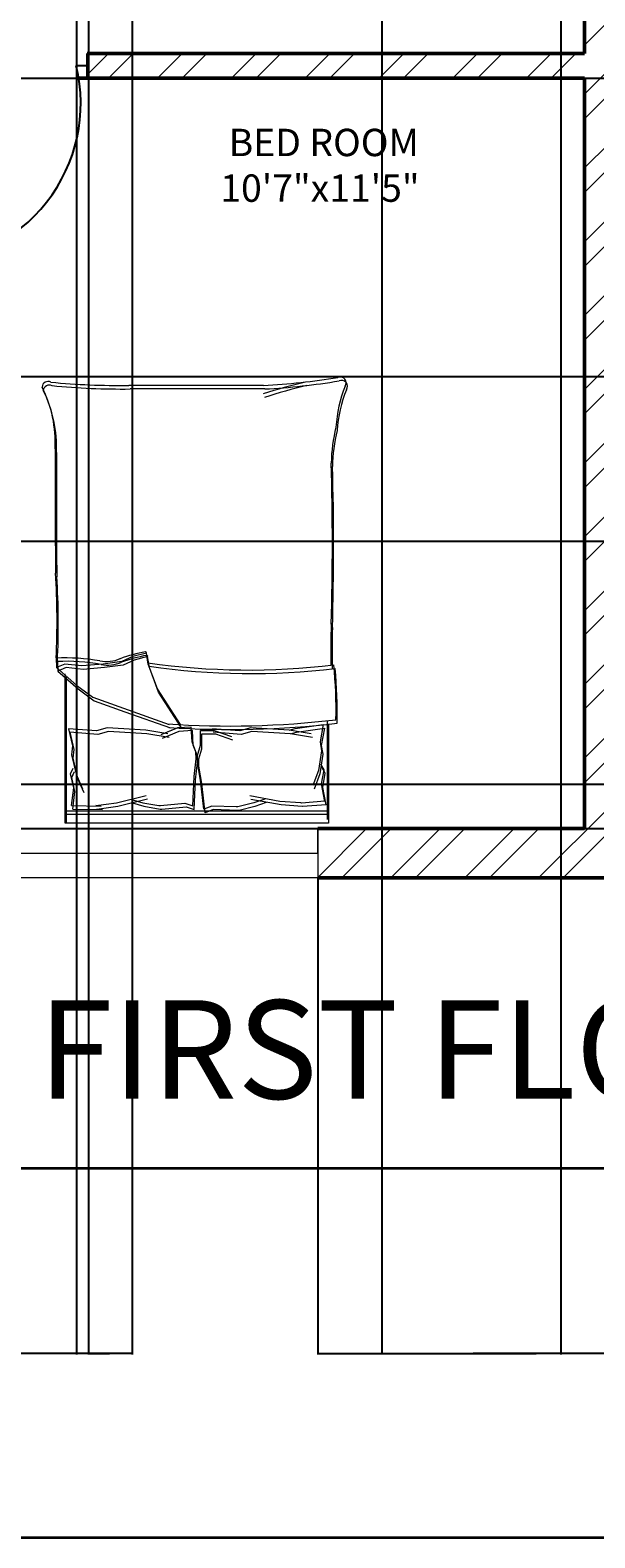
# Model space of a CAD drawing. Units: inches. Extents: x 2310 to 2937, y 1113 to 2410.
# Tile 2 of 23: x 2506 to 2609, y 1616 to 1891. Entities that reach past the tile are written whole.
import ezdxf

# ---------------------------------------------------------------- set-up
doc = ezdxf.new("R2010")
doc.units = ezdxf.units.IN
for name, color, linetype, lineweight in [('A-ANNO-DIMS', 2, 'Continuous', 18), ('A-ANNO-TTLB', 7, 'Continuous', 35), ('A-AREA-IDEN', 7, 'Continuous', 18), ('A-DOOR', 31, 'Continuous', 25), ('A-FURN', 8, 'Continuous', 18), ('A-GLAZ', 191, 'Continuous', 20), ('A-WALL', 7, 'Continuous', 50), ('A-WALL-PATT', 85, 'Continuous', 13)]:
    doc.layers.add(name, color=color, linetype=linetype, lineweight=lineweight)
doc.styles.get("Standard").update_dxf_attribs({"font": 'arial.ttf'})
doc.dimstyles.get("Standard").update_dxf_attribs({"dimtxt": 0.18, "dimasz": 0.18, "dimexe": 0.18, "dimexo": 0.0625, "dimgap": 0.09, "dimtad": 0, "dimtih": 1, "dimtoh": 1, "dimdec": 4, "dimzin": 0, "dimdsep": 46, "dimtxsty": 'Standard', "dimcen": 0.09, "dimadec": 0, "dimazin": 0, "dimtfac": 1, "dimtdec": 4, "dimtofl": 0, "dimtmove": 0, "dimatfit": 3, "dimfxl": 1, "dimtolj": 1, "dimtzin": 0, "dimarcsym": 0})

# ---------------------------------------------------------------- blocks, each defined once
blk = doc.blocks.new('BED-DOUBLE')
for p, q in [((3.56, 63.44), (3.56, 81.55)), ((3.56, 63.44), (3.56, 81.55)), ((3.56, 81.55), (51.58, 81.55)), ((3.56, 80.01), (51.35, 80.01)), ((3.56, 80.01), (51.35, 80.01)), ((3.79, 62.8), (3.79, 80.91)), ((3.79, 62.8), (3.79, 80.91)), ((51.35, 81.55), (51.35, 54.94)), ((51.35, 81.55), (51.35, 54.94)), ((51.58, 81.55), (51.58, 80.91)), ((51.58, 80.91), (51.58, 54.3)), ((51.58, 80.91), (51.58, 54.3)), ((3.79, 79.38), (51.58, 79.38)), ((3.79, 79.38), (51.58, 79.38)), ((3.98, 78.21), (8.27, 78.54)), ((3.98, 78.23), (4.56, 75.05)), ((3.98, 78.23), (4.56, 75.05)), ((3.99, 78.21), (8.27, 78.54)), ((4.21, 77.57), (8.49, 77.9)), ((4.21, 77.57), (8.49, 77.9)), ((4.21, 77.59), (4.79, 74.41)), ((4.21, 77.59), (4.79, 74.41)), ((8.27, 78.54), (8.37, 78.52)), ((8.27, 78.54), (8.37, 78.52)), ((8.37, 78.52), (12.19, 78.23)), ((8.37, 78.52), (12.19, 78.23)), ((8.49, 77.9), (8.6, 77.88)), ((8.49, 77.9), (8.6, 77.88)), ((8.6, 77.88), (12.42, 77.59)), ((8.6, 77.88), (12.42, 77.59)), ((12.19, 78.23), (17.69, 77.22)), ((12.19, 78.23), (17.69, 77.22)), ((12.42, 77.59), (17.92, 76.58)), ((12.42, 77.59), (17.92, 76.58)), ((14.94, 77.8), (16.97, 78.52)), ((14.94, 77.8), (16.96, 78.52)), ((15.17, 77.16), (17.19, 77.88)), ((15.17, 77.16), (17.19, 77.88)), ((16.96, 78.52), (19.86, 79.24)), ((16.97, 78.52), (19.86, 79.24)), ((17.19, 77.88), (20.08, 78.61)), ((17.19, 77.88), (20.08, 78.61)), ((19.86, 79.24), (20.18, 79.24)), ((19.86, 79.24), (20.18, 79.24)), ((20.08, 78.61), (20.41, 78.61)), ((20.08, 78.61), (20.41, 78.61)), ((20.18, 79.24), (24.62, 79.1)), ((20.18, 79.24), (24.62, 79.1)), ((20.41, 78.61), (24.85, 78.46)), ((20.41, 78.61), (24.85, 78.46)), ((24.62, 79.1), (26.07, 79.68)), ((24.62, 79.1), (26.07, 79.68)), ((24.85, 78.46), (26.3, 79.04)), ((24.85, 78.46), (26.3, 79.04)), ((26.07, 79.68), (26.65, 74.33)), ((26.07, 79.68), (26.65, 74.33)), ((26.3, 79.04), (26.88, 73.69)), ((26.3, 79.04), (26.88, 73.69)), ((28.06, 79.06), (27.82, 73.68)), ((28.06, 79.06), (27.82, 73.68)), ((28.29, 78.42), (28.05, 73.04)), ((28.29, 78.42), (28.05, 73.04)), ((29.54, 78.57), (28.06, 79.06)), ((29.54, 78.57), (28.06, 79.06)), ((29.77, 77.93), (28.29, 78.42)), ((29.77, 77.93), (28.29, 78.42)), ((33.97, 78.99), (29.54, 78.57)), ((33.97, 78.99), (29.54, 78.57)), ((34.2, 78.35), (29.77, 77.93)), ((34.2, 78.35), (29.77, 77.93)), ((34.29, 79.01), (33.97, 78.99)), ((34.29, 79.01), (33.97, 78.99)), ((34.52, 78.37), (34.2, 78.35)), ((34.52, 78.37), (34.2, 78.35)), ((37.22, 78.47), (34.29, 79.01)), ((37.22, 78.47), (34.29, 79.01)), ((37.45, 77.83), (34.52, 78.37)), ((37.45, 77.83), (34.52, 78.37)), ((42, 78.48), (36.58, 77.13)), ((42, 78.48), (36.58, 77.13)), ((42.23, 77.84), (36.81, 76.49)), ((42.23, 77.84), (36.81, 76.49)), ((39.29, 77.87), (37.22, 78.47)), ((39.29, 77.87), (37.22, 78.47)), ((39.52, 77.24), (37.45, 77.83)), ((39.51, 77.24), (37.45, 77.83)), ((45.8, 79.01), (42, 78.48)), ((45.8, 79.01), (42, 78.48)), ((46.03, 78.37), (42.23, 77.84)), ((46.03, 78.37), (42.23, 77.84)), ((50.2, 78.99), (44.8, 79.09)), ((44.8, 79.09), (45.8, 79.01)), ((50.2, 78.99), (44.8, 79.09)), ((44.8, 79.09), (45.8, 79.01)), ((50.43, 78.35), (45.02, 78.45)), ((45.02, 78.45), (46.03, 78.37)), ((50.43, 78.35), (45.02, 78.45)), ((45.02, 78.45), (46.03, 78.37)), ((50.2, 78.99), (49.82, 75.78)), ((50.2, 78.99), (49.82, 75.78)), ((50.43, 78.35), (50.05, 75.14)), ((50.43, 78.35), (50.05, 75.14)), ((4.56, 75.05), (4.13, 72.45)), ((4.56, 75.05), (4.13, 72.45)), ((4.79, 74.41), (4.35, 71.81)), ((4.79, 74.41), (4.35, 71.81)), ((5.14, 72.59), (6.15, 75.34)), ((5.14, 72.59), (6.15, 75.34)), ((5.37, 71.95), (6.38, 74.7)), ((5.37, 71.95), (6.38, 74.7)), ((26.65, 74.33), (27.23, 71.15)), ((26.65, 74.33), (27.23, 71.15)), ((49.4, 73.29), (48.21, 75.97)), ((49.4, 73.29), (48.21, 75.97)), ((49.62, 72.65), (48.44, 75.33)), ((49.62, 72.65), (48.44, 75.33)), ((49.82, 75.78), (50.42, 73.21)), ((49.82, 75.78), (50.41, 73.21)), ((50.05, 75.14), (50.64, 72.57)), ((50.05, 75.14), (50.64, 72.57)), ((4.13, 72.45), (4.7, 71.44)), ((4.13, 72.45), (4.7, 71.44)), ((4.35, 71.81), (4.93, 70.8)), ((4.35, 71.81), (4.93, 70.8)), ((4.56, 68.98), (5.14, 72.59)), ((4.56, 68.98), (5.14, 72.59)), ((4.79, 68.34), (5.37, 71.95)), ((4.79, 68.34), (5.37, 71.95)), ((26.88, 73.69), (27.45, 70.51)), ((26.88, 73.69), (27.45, 70.51)), ((27.82, 73.68), (27.44, 70.47)), ((27.82, 73.68), (27.44, 70.47)), ((28.05, 73.04), (27.67, 69.83)), ((28.05, 73.04), (27.67, 69.83)), ((50.2, 69.72), (49.4, 73.29)), ((50.2, 69.72), (49.4, 73.29)), ((50.43, 69.08), (49.62, 72.65)), ((50.43, 69.08), (49.62, 72.65)), ((50.42, 73.21), (49.9, 72.16)), ((50.41, 73.21), (49.9, 72.16)), ((50.64, 72.57), (50.13, 71.52)), ((50.64, 72.57), (50.13, 71.52)), ((4.85, 67.39), (4.56, 68.98)), ((4.85, 67.39), (4.56, 68.98)), ((27.23, 69.85), (26.65, 67.97)), ((27.23, 69.85), (26.65, 67.97)), ((27.45, 69.21), (26.88, 67.33)), ((27.45, 69.21), (26.88, 67.33)), ((27.23, 71.15), (27.23, 69.85)), ((27.23, 71.15), (27.23, 69.85)), ((27.44, 70.47), (27.52, 69.17)), ((27.44, 70.47), (27.52, 69.17)), ((27.45, 70.51), (27.45, 69.21)), ((27.45, 70.51), (27.45, 69.21)), ((27.52, 69.17), (28.22, 67.33)), ((27.52, 69.17), (28.22, 67.33)), ((27.67, 69.83), (27.75, 68.53)), ((27.67, 69.83), (27.75, 68.53)), ((50.01, 68.11), (50.2, 69.72)), ((50.01, 68.11), (50.2, 69.72)), ((50.24, 67.48), (50.43, 69.08)), ((50.24, 67.48), (50.43, 69.08)), ((4.27, 64.21), (4.85, 67.39)), ((4.27, 64.21), (4.85, 67.39)), ((4.5, 63.57), (5.08, 66.75)), ((4.5, 63.57), (5.08, 66.75)), ((5.08, 66.75), (4.79, 68.34)), ((5.08, 66.75), (4.79, 68.34)), ((24.19, 65.29), (21.04, 66.38)), ((24.19, 65.29), (21.05, 66.38)), ((26.65, 67.97), (26.65, 65.29)), ((26.65, 67.97), (26.65, 65.29)), ((26.88, 67.33), (26.88, 64.65)), ((26.88, 67.33), (26.88, 64.65)), ((27.75, 68.53), (28.45, 66.69)), ((27.75, 68.53), (28.44, 66.69)), ((28.22, 67.33), (28.38, 64.66)), ((28.22, 67.33), (28.38, 64.66)), ((28.44, 66.69), (28.61, 64.02)), ((28.45, 66.69), (28.61, 64.02)), ((30.84, 64.81), (33.91, 66.09)), ((30.84, 64.81), (33.91, 66.09)), ((50.78, 64.98), (50.01, 68.11)), ((50.78, 64.98), (50.01, 68.11)), ((51.01, 64.34), (50.24, 67.48)), ((51.01, 64.34), (50.24, 67.48)), ((9.37, 64.93), (4.27, 64.21)), ((9.37, 64.93), (4.27, 64.21)), ((9.6, 64.29), (4.5, 63.57)), ((9.6, 64.29), (4.5, 63.57)), ((6.47, 65.92), (10.5, 65.25)), ((6.47, 65.92), (10.5, 65.25)), ((6.7, 65.28), (10.73, 64.61)), ((6.7, 65.28), (10.73, 64.61)), ((10.5, 65.25), (9.37, 64.93)), ((10.5, 65.25), (9.37, 64.93)), ((10.73, 64.61), (9.6, 64.29)), ((10.73, 64.61), (9.6, 64.29)), ((10.5, 65.25), (17.51, 64.82)), ((10.5, 65.25), (17.51, 64.82)), ((10.73, 64.61), (17.74, 64.18)), ((10.73, 64.61), (17.74, 64.18)), ((17.51, 64.82), (19.47, 65.38)), ((17.51, 64.82), (19.47, 65.38)), ((17.74, 64.18), (19.7, 64.74)), ((17.74, 64.18), (19.7, 64.74)), ((19.47, 65.38), (24.6, 64.98)), ((19.47, 65.38), (24.6, 64.98)), ((19.7, 64.74), (24.83, 64.34)), ((19.7, 64.74), (24.83, 64.34)), ((24.42, 64.65), (21.27, 65.74)), ((24.42, 64.65), (21.27, 65.74)), ((26.65, 65.29), (24.19, 65.29)), ((26.65, 65.29), (24.19, 65.29)), ((26.88, 64.65), (24.42, 64.65)), ((26.88, 64.65), (24.42, 64.65)), ((28.38, 64.66), (30.84, 64.81)), ((28.38, 64.66), (30.84, 64.81)), ((28.61, 64.02), (31.07, 64.17)), ((28.61, 64.02), (31.06, 64.17)), ((30.35, 64.17), (34.54, 57.67)), ((30.35, 64.17), (34.54, 57.67)), ((30.57, 63.53), (34.76, 57.03)), ((30.57, 63.53), (34.76, 57.03)), ((31.06, 64.17), (34.14, 65.45)), ((31.07, 64.17), (34.14, 65.45)), ((40.73, 61.23), (32.39, 64.17)), ((40.73, 61.23), (32.39, 64.17)), ((40.96, 60.59), (32.62, 63.53)), ((40.96, 60.59), (32.62, 63.53)), ((32.65, 65.92), (36.68, 65.25)), ((32.65, 65.92), (36.68, 65.25)), ((32.88, 65.28), (36.91, 64.61)), ((32.88, 65.28), (36.91, 64.61)), ((36.68, 65.25), (43.69, 64.82)), ((36.68, 65.25), (43.69, 64.82)), ((36.91, 64.61), (43.92, 64.18)), ((36.91, 64.61), (43.92, 64.18)), ((43.69, 64.82), (45.65, 65.38)), ((43.69, 64.82), (45.65, 65.38)), ((43.92, 64.18), (45.88, 64.74)), ((43.92, 64.18), (45.88, 64.74)), ((45.65, 65.38), (50.78, 64.98)), ((45.65, 65.38), (50.78, 64.98)), ((45.88, 64.74), (51.01, 64.34)), ((45.88, 64.74), (51.01, 64.34)), ((46.31, 59.22), (40.73, 61.23)), ((46.31, 59.22), (40.73, 61.23)), ((46.53, 58.58), (40.96, 60.59)), ((46.53, 58.58), (40.96, 60.59)), ((49.25, 57.05), (46.31, 59.22)), ((49.25, 57.05), (46.31, 59.22)), ((49.48, 56.41), (46.53, 58.58)), ((49.48, 56.41), (46.53, 58.58)), ((34.54, 57.67), (36.24, 53.18)), ((34.54, 57.67), (36.24, 53.18)), ((34.76, 57.03), (36.47, 52.54)), ((34.76, 57.03), (36.47, 52.54)), ((52.95, 53.8), (49.25, 57.05)), ((52.95, 53.8), (49.25, 57.05)), ((53.18, 53.16), (49.48, 56.41)), ((53.18, 53.16), (49.48, 56.41)), ((36.24, 53.18), (36.55, 51.17)), ((36.24, 53.18), (36.55, 51.17)), ((36.47, 52.54), (36.78, 50.53)), ((36.47, 52.54), (36.78, 50.53)), ((39.03, 51.79), (41.04, 52.72)), ((39.03, 51.79), (41.04, 52.72)), ((41.04, 52.72), (44.45, 53.18)), ((41.04, 52.72), (44.45, 53.18)), ((41.27, 52.08), (44.68, 52.54)), ((41.27, 52.08), (44.68, 52.54)), ((44.45, 53.18), (48.32, 53.49)), ((44.45, 53.18), (48.32, 53.49)), ((44.68, 52.54), (48.55, 52.85)), ((44.68, 52.54), (48.55, 52.85)), ((48.32, 53.49), (51.42, 53.18)), ((48.32, 53.49), (51.42, 53.18)), ((48.55, 52.85), (51.65, 52.54)), ((48.55, 52.85), (51.65, 52.54)), ((51.42, 53.18), (52.95, 53.8)), ((51.42, 53.18), (52.95, 53.8)), ((51.65, 52.54), (53.18, 53.16)), ((51.65, 52.54), (53.18, 53.16)), ((53.03, 52.06), (52.95, 53.8, 3.87)), ((53.03, 52.06), (52.95, 53.8, 3.87)), ((53.26, 51.42), (53.18, 53.16, 3.87)), ((53.26, 51.42), (53.18, 53.16, 3.87)), ((36.55, 51.17), (39.03, 51.79)), ((36.55, 51.17), (39.03, 51.79)), ((36.78, 50.53), (39.26, 51.15)), ((36.78, 50.53), (39.26, 51.15)), ((39.26, 51.15), (41.27, 52.08)), ((39.26, 51.15), (41.27, 52.08)), ((15.15, 2.3), (39.76, 2.3)), ((15.15, 2.3), (39.76, 2.3)), ((15.38, 1.66), (39.99, 1.66)), ((15.38, 1.66), (39.99, 1.66))]:
    blk.add_line(p, q)
for centre, radius, start, end in [((85.25, 61.45), 83.31, 178.7218, 185.604), ((85.25, 61.45), 83.31, 178.7218, 185.604), ((21.45, -100.5), 164.97, 86.0865, 96.7821), ((21.45, -100.5), 164.97, 86.0865, 96.7821), ((21.67, -101.14), 164.97, 86.0865, 96.7821), ((21.67, -101.14), 164.97, 86.0865, 96.7821), ((85.48, 60.81), 83.31, 178.7218, 185.604), ((85.48, 60.81), 83.31, 178.7218, 185.604), ((17.84, -74.77), 129.02, 81.7845, 96.9006), ((17.84, -74.77), 129.02, 81.7845, 96.9006), ((18.07, -75.41), 129.02, 81.7845, 96.9006), ((18.07, -75.41), 129.02, 81.7845, 96.9006), ((-167.22, 50.37), 170.11, 358.4762, 1.0082), ((-167.22, 50.37), 170.11, 358.4762, 1.0082), ((-166.99, 49.74), 170.11, 358.4762, 1.0082), ((-166.99, 49.74), 170.11, 358.4762, 1.0082), ((43.83, 46.48), 6.22, 78.6608, 113.7384), ((43.83, 46.48), 6.22, 78.6608, 113.7384), ((51.41, 88.2), 36.18, 259.8763, 272.5657), ((51.41, 88.2), 36.18, 259.8763, 272.5657), ((36.72, 51.11), 0.185, 160.2464, 271.1377), ((36.72, 51.11), 0.185, 160.2464, 271.1377), ((31.24, 80.07), 29.65, 280.6617, 289.8806), ((31.24, 80.07), 29.65, 280.6617, 289.8806), ((36.95, 50.47), 0.185, 160.2464, 271.1377), ((36.95, 50.47), 0.185, 160.2464, 271.1377), ((31.47, 79.43), 29.65, 280.6617, 289.8806), ((31.47, 79.43), 29.65, 280.6617, 289.8806), ((44.06, 45.84), 6.22, 78.6608, 113.7384), ((44.06, 45.84), 6.22, 78.6608, 113.7384), ((51.64, 87.57), 36.18, 259.8763, 272.5657), ((51.64, 87.57), 36.18, 259.8763, 272.5657), ((182.35, 45.23), 129.5, 176.9791, 183.8365), ((182.35, 45.23), 129.5, 176.9791, 183.8365), ((182.58, 44.59), 129.5, 176.9791, 183.8365), ((182.58, 44.59), 129.5, 176.9791, 183.8365), ((484.91, 30.93), 482.31, 178.2277, 181.7185), ((484.91, 30.93), 482.31, 178.2277, 181.7185), ((485.14, 30.3), 482.31, 178.2277, 181.7185), ((485.14, 30.3), 482.31, 178.2277, 181.7185), ((-4508.66, 13.73), 4561.86, 0.00217, 0.28689), ((-4508.66, 13.73), 4561.86, 0.00217, 0.28689), ((-4508.43, 13.09), 4561.86, 0.00217, 0.28689), ((-4508.43, 13.09), 4561.86, 0.00217, 0.28689), ((-26.81, 17.03), 29.63, 346.0648, 358.9113), ((-26.81, 17.03), 29.63, 346.0648, 358.9113), ((-26.58, 16.39), 29.63, 346.0648, 358.9113), ((-26.58, 16.39), 29.63, 346.0648, 358.9113), ((76.24, 12.88), 23.07, 177.4714, 206.4681), ((76.24, 12.88), 23.07, 177.4714, 206.4681), ((76.47, 12.24), 23.07, 177.4714, 206.4681), ((76.47, 12.24), 23.07, 177.4714, 206.4681), ((-21.57, 11.27), 23.56, 337.9751, 356.652), ((-21.57, 11.27), 23.56, 337.9751, 356.652), ((-21.34, 10.63), 23.56, 337.9751, 356.652), ((-21.34, 10.63), 23.56, 337.9751, 356.652), ((-17.14, 105.26), 106.46, 283.3832, 287.7053), ((-17.14, 105.26), 106.46, 283.3832, 287.7053), ((-16.91, 104.62), 106.46, 283.3832, 287.7053), ((-16.91, 104.62), 106.46, 283.3832, 287.7053), ((1.17, 1.83), 1.09, 146.1736, 293.4781), ((1.17, 1.83), 1.09, 146.1736, 293.4781), ((1.4, 1.19), 1.09, 146.1736, 293.4781), ((1.4, 1.19), 1.09, 146.1736, 293.4781), ((21.51, -119.29), 121.76, 92.9958, 99.4091), ((21.51, -119.29), 121.76, 92.9958, 99.4091), ((21.74, -119.93), 121.76, 92.9958, 99.4091), ((21.74, -119.93), 121.76, 92.9958, 99.4091), ((41.24, -130.73), 133.04, 84.4998, 90.6351), ((41.24, -130.73), 133.04, 84.4998, 90.6351), ((41.47, -131.37), 133.04, 84.4998, 90.6351), ((41.47, -131.37), 133.04, 84.4998, 90.6351), ((54.5, 2.68), 1.1, 242.6588, 356.02), ((54.5, 2.68), 1.1, 242.6588, 356.02), ((54.72, 2.04), 1.1, 242.6588, 356.02), ((54.72, 2.04), 1.1, 242.6588, 356.02)]:
    blk.add_arc(centre, radius, start, end)
blk = doc.blocks.new('WIN-60IN')
for p, q in [((4.5, 60), (0, 60)), ((0, 60), (9, 60)), ((0, 60), (0, 0)), ((4.5, 0), (4.5, 60)), ((9, 60), (9, 0)), ((0, 0), (9, 0)), ((9, 0), (4.5, 0))]:
    blk.add_line(p, q)
blk = doc.blocks.new('*D44')
at = {"layer": 'A-ANNO-DIMS', "color": 0, "lineweight": -2, "transparency": 16777216}
for p, q in [((2558.31, 1736.45), (2558.31, 1649.5)), ((2638.89, 1736.45), (2638.89, 1649.5)), ((2558.49, 1649.68), (2598.21, 1649.68)), ((2638.71, 1649.68), (2598.99, 1649.68))]:
    blk.add_line(p, q, dxfattribs=at)
at = {"layer": 'A-ANNO-DIMS', "color": 0, "transparency": 16777216}
for points in [[(2558.49, 1649.71), (2558.49, 1649.65), (2558.31, 1649.68)], [(2638.71, 1649.71), (2638.71, 1649.65), (2638.89, 1649.68)]]:
    blk.add_solid(points, dxfattribs=at)
at = {"layer": 'Defpoints', "color": 0, "transparency": 16777216}
for p in [(2558.31, 1736.51), (2638.89, 1736.51), (2638.89, 1649.68)]:
    blk.add_point(p, dxfattribs=at)
at = {"layer": 'A-ANNO-DIMS', "color": 0, "transparency": 16777216, "insert": (2598.6, 1649.68), "char_height": 0.18, "attachment_point": 5}
blk.add_mtext('\\A1;80.59', dxfattribs=at)
blk = doc.blocks.new('*D55')
at = {"layer": 'A-ANNO-DIMS', "color": 0, "lineweight": -2, "transparency": 16777216}
for p, q in [((2403.55, 1753.64), (2858.02, 1753.64)), ((2857.84, 1753.46), (2857.84, 1749.76)), ((2857.84, 1745.69), (2857.84, 1749.4)), ((2403.55, 1745.51), (2858.02, 1745.51))]:
    blk.add_line(p, q, dxfattribs=at)
at = {"layer": 'A-ANNO-DIMS', "color": 0, "transparency": 16777216}
for points in [[(2857.81, 1753.46), (2857.87, 1753.46), (2857.84, 1753.64)], [(2857.81, 1745.69), (2857.87, 1745.69), (2857.84, 1745.51)]]:
    blk.add_solid(points, dxfattribs=at)
at = {"layer": 'Defpoints', "color": 0, "transparency": 16777216}
for p in [(2403.49, 1753.64), (2857.84, 1753.64), (2403.49, 1745.51)]:
    blk.add_point(p, dxfattribs=at)
at = {"layer": 'A-ANNO-DIMS', "color": 0, "transparency": 16777216, "insert": (2857.84, 1749.58), "char_height": 0.18, "attachment_point": 5}
blk.add_mtext('\\A1;8.127', dxfattribs=at)
blk = doc.blocks.new('*D56')
at = {"layer": 'A-ANNO-DIMS', "color": 0, "lineweight": -2, "transparency": 16777216}
for p, q in [((2403.55, 1828.04), (2858.02, 1828.04)), ((2857.84, 1827.86), (2857.84, 1813.21)), ((2857.84, 1798.19), (2857.84, 1812.85)), ((2403.55, 1798.01), (2858.02, 1798.01))]:
    blk.add_line(p, q, dxfattribs=at)
at = {"layer": 'A-ANNO-DIMS', "color": 0, "transparency": 16777216}
for points in [[(2857.81, 1827.86), (2857.87, 1827.86), (2857.84, 1828.04)], [(2857.81, 1798.19), (2857.87, 1798.19), (2857.84, 1798.01)]]:
    blk.add_solid(points, dxfattribs=at)
at = {"layer": 'Defpoints', "color": 0, "transparency": 16777216}
for p in [(2403.49, 1828.04), (2857.84, 1828.04), (2403.49, 1798.01)]:
    blk.add_point(p, dxfattribs=at)
at = {"layer": 'A-ANNO-DIMS', "color": 0, "transparency": 16777216, "insert": (2857.84, 1813.03), "char_height": 0.18, "attachment_point": 5}
blk.add_mtext('\\A1;30.03', dxfattribs=at)
blk = doc.blocks.new('*D58')
at = {"layer": 'A-ANNO-DIMS', "color": 0, "lineweight": -2, "transparency": 16777216}
for p, q in [((2475.55, 1882.51), (2858.02, 1882.51)), ((2857.84, 1882.33), (2857.84, 1840.45)), ((2857.84, 1798.19), (2857.84, 1840.08)), ((2475.55, 1798.01), (2858.02, 1798.01))]:
    blk.add_line(p, q, dxfattribs=at)
at = {"layer": 'A-ANNO-DIMS', "color": 0, "transparency": 16777216}
for points in [[(2857.81, 1882.33), (2857.87, 1882.33), (2857.84, 1882.51)], [(2857.81, 1798.19), (2857.87, 1798.19), (2857.84, 1798.01)]]:
    blk.add_solid(points, dxfattribs=at)
at = {"layer": 'Defpoints', "color": 0, "transparency": 16777216}
for p in [(2475.49, 1882.51), (2857.84, 1882.51), (2475.49, 1798.01)]:
    blk.add_point(p, dxfattribs=at)
at = {"layer": 'A-ANNO-DIMS', "color": 0, "transparency": 16777216, "insert": (2857.84, 1840.26), "char_height": 0.18, "attachment_point": 5}
blk.add_mtext('\\A1;84.5', dxfattribs=at)
blk = doc.blocks.new('*D61')
at = {"layer": 'A-ANNO-DIMS', "color": 0, "lineweight": -2, "transparency": 16777216}
for p, q in [((2484.33, 2205.95), (2484.33, 1649.5)), ((2514.27, 2205.95), (2514.27, 1649.5)), ((2484.51, 1649.68), (2498.9, 1649.68)), ((2514.09, 1649.68), (2499.69, 1649.68))]:
    blk.add_line(p, q, dxfattribs=at)
at = {"layer": 'A-ANNO-DIMS', "color": 0, "transparency": 16777216}
for points in [[(2484.51, 1649.71), (2484.51, 1649.65), (2484.33, 1649.68)], [(2514.09, 1649.71), (2514.09, 1649.65), (2514.27, 1649.68)]]:
    blk.add_solid(points, dxfattribs=at)
at = {"layer": 'Defpoints', "color": 0, "transparency": 16777216}
for p in [(2484.33, 2206.01), (2514.27, 2206.01), (2514.27, 1649.68)]:
    blk.add_point(p, dxfattribs=at)
at = {"layer": 'A-ANNO-DIMS', "color": 0, "transparency": 16777216, "insert": (2499.3, 1649.68), "char_height": 0.18, "attachment_point": 5}
blk.add_mtext('\\A1;29.94', dxfattribs=at)
blk = doc.blocks.new('*D62')
at = {"layer": 'A-ANNO-DIMS', "color": 0, "lineweight": -2, "transparency": 16777216}
for p, q in [((2569.99, 2093.45), (2569.99, 1649.5)), ((2602.69, 2093.45), (2602.69, 1649.5)), ((2570.17, 1649.68), (2586.02, 1649.68)), ((2602.51, 1649.68), (2586.66, 1649.68))]:
    blk.add_line(p, q, dxfattribs=at)
at = {"layer": 'A-ANNO-DIMS', "color": 0, "transparency": 16777216}
for points in [[(2570.17, 1649.71), (2570.17, 1649.65), (2569.99, 1649.68)], [(2602.51, 1649.71), (2602.51, 1649.65), (2602.69, 1649.68)]]:
    blk.add_solid(points, dxfattribs=at)
at = {"layer": 'Defpoints', "color": 0, "transparency": 16777216}
for p in [(2569.99, 2093.51), (2602.69, 2093.51), (2602.69, 1649.68)]:
    blk.add_point(p, dxfattribs=at)
at = {"layer": 'A-ANNO-DIMS', "color": 0, "transparency": 16777216, "insert": (2586.34, 1649.68), "char_height": 0.18, "attachment_point": 5}
blk.add_mtext('\\A1;32.7', dxfattribs=at)
blk = doc.blocks.new('*D63')
at = {"layer": 'A-ANNO-DIMS', "color": 0, "lineweight": -2, "transparency": 16777216}
for p, q in [((2436.46, 1999.45), (2436.46, 1649.5)), ((2524.46, 1999.45), (2524.46, 1649.5)), ((2436.64, 1649.68), (2480.25, 1649.68)), ((2524.28, 1649.68), (2480.68, 1649.68))]:
    blk.add_line(p, q, dxfattribs=at)
at = {"layer": 'A-ANNO-DIMS', "color": 0, "transparency": 16777216}
for points in [[(2436.64, 1649.71), (2436.64, 1649.65), (2436.46, 1649.68)], [(2524.28, 1649.71), (2524.28, 1649.65), (2524.46, 1649.68)]]:
    blk.add_solid(points, dxfattribs=at)
at = {"layer": 'Defpoints', "color": 0, "transparency": 16777216}
for p in [(2436.46, 1999.51), (2524.46, 1999.51), (2524.46, 1649.68)]:
    blk.add_point(p, dxfattribs=at)
at = {"layer": 'A-ANNO-DIMS', "color": 0, "transparency": 16777216, "insert": (2480.46, 1649.68), "char_height": 0.18, "attachment_point": 5}
blk.add_mtext('\\A1;88', dxfattribs=at)
blk = doc.blocks.new('*D66')
at = {"layer": 'A-ANNO-DIMS', "color": 0, "lineweight": -2, "transparency": 16777216}
for p, q in [((2516.46, 2093.45), (2516.46, 1649.5)), ((2524.46, 2093.45), (2524.46, 1649.5)), ((2516.64, 1649.68), (2520.32, 1649.68)), ((2524.28, 1649.68), (2520.61, 1649.68))]:
    blk.add_line(p, q, dxfattribs=at)
at = {"layer": 'A-ANNO-DIMS', "color": 0, "transparency": 16777216}
for points in [[(2516.64, 1649.71), (2516.64, 1649.65), (2516.46, 1649.68)], [(2524.28, 1649.71), (2524.28, 1649.65), (2524.46, 1649.68)]]:
    blk.add_solid(points, dxfattribs=at)
at = {"layer": 'Defpoints', "color": 0, "transparency": 16777216}
for p in [(2516.46, 2093.51), (2524.46, 2093.51), (2524.46, 1649.68)]:
    blk.add_point(p, dxfattribs=at)
at = {"layer": 'A-ANNO-DIMS', "color": 0, "transparency": 16777216, "insert": (2520.46, 1649.68), "char_height": 0.18, "attachment_point": 5}
blk.add_mtext('\\A1;8', dxfattribs=at)

msp = doc.modelspace()

# ---------------------------------------------------------------- hatches: boundary and pattern name
at = {"layer": 'A-WALL-PATT'}
h = msp.add_hatch(dxfattribs=at)
h.set_pattern_fill('ANSI32', color=256)
h.paths.add_polyline_path([(2639.1394, 2356.5139), (2563.662, 2356.5139), (2563.662, 2347.5139), (2606.9859, 2347.5139), (2606.9859, 2210.5139), (2514.2692, 2210.5139), (2514.2692, 2206.0139), (2606.9859, 2206.0139), (2606.9859, 2098.0139), (2602.689, 2098.0139), (2602.689, 2093.5139), (2615.5262, 2093.5139), (2615.5262, 2095.7639), (2615.5262, 2098.0139), (2611.4859, 2098.0139), (2611.4859, 2206.0139), (2703.9391, 2206.0139), (2703.9391, 2208.2639), (2703.9391, 2210.5139), (2611.4859, 2210.5139), (2611.4859, 2347.5139), (2639.1394, 2347.5139)])
h.paths.add_polyline_path([(2823.9859, 2356.5139), (2699.1394, 2356.5139), (2699.1394, 2347.5139), (2738.4859, 2347.5139), (2738.4859, 2343.9266), (2742.9859, 2343.9266), (2742.9859, 2347.5139), (2814.9859, 2347.5139), (2814.9859, 2336.76), (2823.9859, 2336.76)])
h.paths.add_polyline_path([(2823.9859, 2312.76), (2814.9859, 2312.76), (2814.9859, 2299.5139), (2742.9859, 2299.5139), (2742.9859, 2323.0159), (2740.7359, 2323.0159), (2738.4859, 2323.0159), (2738.4859, 2210.5139), (2734.5483, 2210.5139), (2734.5483, 2206.0139), (2746.8769, 2206.0139), (2746.8769, 2208.2639), (2746.8769, 2210.5139), (2742.9859, 2210.5139), (2742.9859, 2295.0139), (2814.9859, 2295.0139), (2814.9859, 2269.8977), (2823.9859, 2269.8977)])
h.paths.add_polyline_path([(2823.9859, 2210.5139), (2823.9859, 2233.8977), (2819.4859, 2233.8977), (2814.9859, 2233.8977), (2814.9859, 2210.5139), (2769.9745, 2210.5139), (2769.9745, 2206.0139), (2814.9859, 2206.0139), (2814.9859, 2178.3027), (2823.9859, 2178.3027)])
h.paths.add_polyline_path([(2823.9859, 2118.3027), (2819.4859, 2118.3027), (2814.9859, 2118.3027), (2814.9859, 2098.0139), (2647.0333, 2098.0139), (2647.0333, 2093.5139), (2814.9859, 2093.5139), (2814.9859, 1999.5139), (2650.6052, 1999.5139), (2650.6052, 1995.0139), (2814.9859, 1995.0139), (2814.9859, 1969.9784), (2823.9859, 1969.9784)])
h.paths.add_polyline_path([(2403.4859, 2093.5139), (2569.9888, 2093.5139), (2569.9888, 2095.7639), (2569.9888, 2098.0139), (2403.4859, 2098.0139), (2403.4859, 2131.7587), (2394.4859, 2131.7587), (2394.4859, 1967.522), (2403.4859, 1967.522), (2403.4859, 1995.0139), (2569.8903, 1995.0139), (2569.8903, 1997.2639), (2569.8903, 1999.5139), (2403.4859, 1999.5139)])
h.paths.add_polyline_path([(2503.662, 2356.5139), (2394.4859, 2356.5139), (2394.4859, 2337.9231), (2398.9859, 2337.9231), (2403.4859, 2337.9231), (2403.4859, 2347.5139), (2475.4859, 2347.5139), (2475.4859, 2343.0384), (2479.9859, 2343.0384), (2479.9859, 2347.5139), (2503.662, 2347.5139)])
h.paths.add_polyline_path([(2498.3065, 1745.5139), (2479.9859, 1745.5139), (2479.9859, 1749.1663), (2477.7359, 1749.1663), (2475.4859, 1749.1663), (2475.4859, 1745.5139), (2403.4859, 1745.5139), (2403.4859, 1753.6409), (2398.9859, 1753.6409), (2394.4859, 1753.6409), (2394.4859, 1736.5139), (2498.3065, 1736.5139), (2498.3065, 1741.0139)])
h.paths.add_polyline_path([(2479.9859, 1882.5139), (2483.9367, 1882.5139), (2483.9367, 1887.0139), (2471.5501, 1887.0139), (2471.5501, 1885.1969), (2471.5501, 1882.5139), (2475.4859, 1882.5139), (2475.4859, 1798.0139), (2403.4859, 1798.0139), (2403.4859, 1828.0433), (2402.2852, 1828.0433), (2394.4859, 1828.0433), (2394.4859, 1777.6409), (2403.4859, 1777.6409), (2403.4859, 1793.5139), (2475.4859, 1793.5139), (2475.4859, 1769.1696), (2479.9859, 1769.1696)])
h.paths.add_polyline_path([(2403.4859, 1907.522), (2398.9859, 1907.522), (2394.4859, 1907.522), (2394.4859, 1864.0433), (2403.4859, 1864.0433), (2403.4859, 1882.5139), (2448.9325, 1882.5139), (2448.9325, 1884.7639), (2448.9325, 1887.0139), (2403.4859, 1887.0139)])
h.paths.add_polyline_path([(2702.2061, 1887.0139), (2611.4859, 1887.0139), (2611.4859, 1995.0139), (2615.6132, 1995.0139), (2615.6132, 1999.5139), (2602.4798, 1999.5139), (2602.4798, 1997.2639), (2602.4798, 1995.0139), (2606.9859, 1995.0139), (2606.9859, 1887.0139), (2516.2443, 1887.0139), (2516.2443, 1884.7639), (2516.2443, 1882.5139), (2606.9859, 1882.5139), (2606.9859, 1745.5139), (2558.3065, 1745.5139), (2558.3065, 1736.5139), (2638.8921, 1736.5139), (2638.8921, 1741.0139), (2638.8921, 1745.5139), (2611.4859, 1745.5139), (2611.4859, 1882.5139), (2702.2061, 1882.5139)])
h.paths.add_polyline_path([(2823.9859, 1909.9784), (2819.4859, 1909.9784), (2814.9859, 1909.9784), (2814.9859, 1887.0139), (2769.144, 1887.0139), (2769.144, 1884.7639), (2769.144, 1882.5139), (2814.9859, 1882.5139), (2814.9859, 1854.1704), (2823.9859, 1854.1704)])
h.paths.add_polyline_path([(2823.9859, 1818.1704), (2819.4859, 1818.1704), (2814.9859, 1818.1704), (2814.9859, 1798.0139), (2742.9859, 1798.0139), (2742.9859, 1882.5139), (2746.805, 1882.5139), (2746.805, 1887.0139), (2733.7334, 1887.0139), (2733.7334, 1884.7639), (2733.7334, 1882.5139), (2738.4859, 1882.5139), (2738.4859, 1771.1728), (2740.7359, 1771.1728), (2742.9859, 1771.1728), (2742.9859, 1793.5139), (2814.9859, 1793.5139), (2814.9859, 1783.6684), (2823.9859, 1783.6684)])
h.paths.add_polyline_path([(2823.9859, 1759.6684), (2814.9859, 1759.6684), (2814.9859, 1745.5139), (2742.9859, 1745.5139), (2742.9859, 1748.9831), (2740.7359, 1748.9831), (2738.4859, 1748.9831), (2738.4859, 1745.5139), (2698.8921, 1745.5139), (2698.8921, 1736.5139), (2823.9859, 1736.5139)])

# ---------------------------------------------------------------- linework, layer by layer
at = {"layer": 'A-ANNO-TTLB'}
msp.add_line((2487.6418, 1683.5307), (2761.8399, 1683.5307), dxfattribs=at)
msp.add_lwpolyline([(2310.2498, 2409.8427), (2937.0534, 2409.8427), (2937.0534, 1616.036), (2310.2498, 1616.036)], close=True, dxfattribs=at)
at = {"layer": 'A-DOOR'}
for p, q in [((2516.2443, 1882.5139), (2516.2443, 1887.0139)), ((2516.2443, 1887.0139), (2516.2443, 1884.7639)), ((2516.2443, 1884.7639), (2514.2443, 1884.7639))]:
    msp.add_line(p, q, dxfattribs=at)
msp.add_arc((2485.9367, 1877.8934), 29.1295, 270, 13.642354, dxfattribs=at)
at = {"layer": 'A-WALL'}
for p, q in [((2606.9859, 1995.0139), (2606.9859, 1887.0139)), ((2516.2443, 1887.0139), (2606.9859, 1887.0139)), ((2514.6974, 1882.5139), (2606.9859, 1882.5139)), ((2606.9859, 1882.5139), (2606.9859, 1745.5139)), ((2558.3065, 1745.5139), (2606.9859, 1745.5139)), ((2558.3065, 1736.5139), (2638.8921, 1736.5139))]:
    msp.add_line(p, q, dxfattribs=at)

# ---------------------------------------------------------------- block references
at = {"layer": 'A-FURN', "rotation": 180}
msp.add_blockref('BED-DOUBLE', (2563.8198, 1828.0743), dxfattribs=at)
at = {"layer": 'A-GLAZ', "rotation": 270}
msp.add_blockref('WIN-60IN', (2498.3065, 1745.5139), dxfattribs=at)

# ---------------------------------------------------------------- texts
at = {"layer": 'A-ANNO-TTLB', "insert": (2507.293, 1714.1887), "char_height": 18, "attachment_point": 1}
msp.add_mtext_dynamic_manual_height_columns('FIRST FLOOR PLAN', width=651.219844, gutter_width=12.5, heights=[0], dxfattribs=at)
at = {"layer": 'A-AREA-IDEN', "insert": (2529.8366, 1873.2722), "char_height": 5, "attachment_point": 1}
msp.add_mtext_dynamic_manual_height_columns('        BED ROOM\\P       10\'7"x11\'5"', width=232.117602, gutter_width=12.5, heights=[0], dxfattribs=at)

# ---------------------------------------------------------------- dimensions: what is measured, and where the dimension line sits
at = {"layer": 'A-ANNO-DIMS'}
for base, p1, p2, override, picture, middle in [((2514.2692, 1649.6807), (2484.3278, 2206.0139), (2514.2692, 2206.0139), {"dimdec": 2, "dimlfac": 1, "dimrnd": 0, "dimzin": 0, "dimdsep": 46, "dimlunit": 2}, '*D61', (2499.2985, 1649.6807)), ((2524.4647, 1649.6807), (2516.4647, 2093.5139), (2524.4647, 2093.5139), {"dimdec": 0, "dimlfac": 1, "dimrnd": 0, "dimzin": 0, "dimdsep": 46, "dimlunit": 2}, '*D66', (2520.4647, 1649.6807)), ((2602.689, 1649.6807), (2569.9888, 2093.5139), (2602.689, 2093.5139), {"dimdec": 1, "dimlfac": 1, "dimrnd": 0, "dimzin": 0, "dimdsep": 46, "dimlunit": 2}, '*D62', (2586.3389, 1649.6807)), ((2524.4647, 1649.6807), (2436.4647, 1999.5139), (2524.4647, 1999.5139), {"dimdec": 0, "dimlfac": 1, "dimrnd": 0, "dimzin": 0, "dimdsep": 46, "dimlunit": 2}, '*D63', (2480.4647, 1649.6807)), ((2638.8921, 1649.6807), (2558.3065, 1736.5139), (2638.8921, 1736.5139), {"dimdec": 2, "dimlfac": 1, "dimrnd": 0, "dimzin": 0, "dimdsep": 46, "dimlunit": 2}, '*D44', (2598.5993, 1649.6807))]:
    dim = msp.add_linear_dim(base=base, p1=p1, p2=p2, dimstyle='Standard', override=override, dxfattribs=at)
    dim.commit()
    dim.dimension.update_dxf_attribs({"geometry": picture, "text_midpoint": middle})
for base, p1, p2, override, picture, middle in [((2857.8359, 1882.5139), (2475.4859, 1798.0139), (2475.4859, 1882.5139), {"dimdec": 1, "dimlfac": 1, "dimrnd": 0, "dimzin": 0, "dimdsep": 46, "dimlunit": 2}, '*D58', (2857.8359, 1840.2639)), ((2857.8359, 1828.0433), (2403.4859, 1798.0139), (2403.4859, 1828.0433), {"dimdec": 2, "dimlfac": 1, "dimrnd": 0, "dimzin": 0, "dimdsep": 46, "dimlunit": 2}, '*D56', (2857.8359, 1813.0286)), ((2857.8359, 1753.6409), (2403.4859, 1745.5139), (2403.4859, 1753.6409), {"dimdec": 3, "dimlfac": 1, "dimrnd": 0, "dimzin": 0, "dimdsep": 46, "dimlunit": 2}, '*D55', (2857.8359, 1749.5774))]:
    dim = msp.add_linear_dim(base=base, p1=p1, p2=p2, angle=90, dimstyle='Standard', override=override, dxfattribs=at)
    dim.commit()
    dim.dimension.update_dxf_attribs({"geometry": picture, "text_midpoint": middle})

doc.saveas('drawing.dxf')
